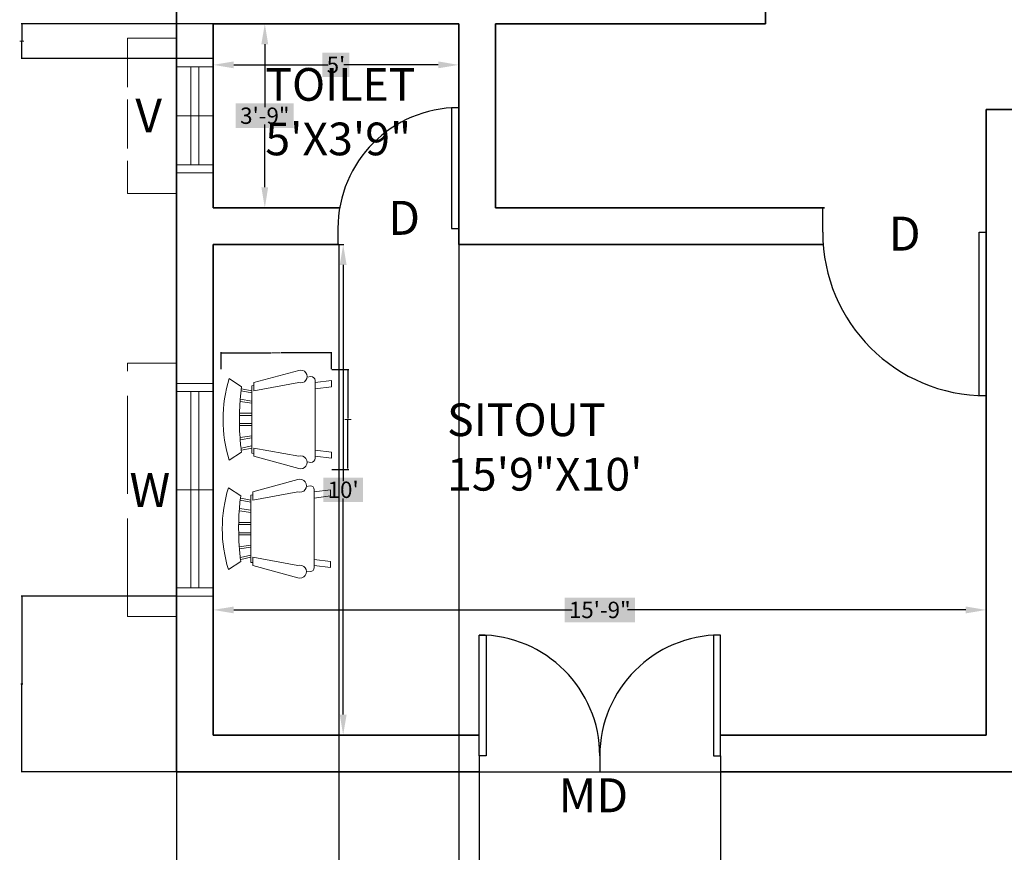
# Model space of a CAD drawing. Units: inches. Extents: x -128 to 854, y -395 to 398.
# Tile 22 of 61: x -88 to 152, y -109 to 95. Entities that reach past the tile are written whole.
import ezdxf

# ---------------------------------------------------------------- set-up
doc = ezdxf.new("R2010")
doc.units = ezdxf.units.IN
doc.header["$MEASUREMENT"] = 0
doc.linetypes.add('ACAD_ISO02W100', pattern=[15, 12, -3])
for name, color, linetype, lineweight in [('A-ANNO-DIMS', 2, 'Continuous', 18), ('A-ANNO-TEXT', 2, 'Continuous', 18), ('A-AREA-IDEN', 1, 'Continuous', 18), ('A-DOOR', 4, 'Continuous', 25), ('A-FURN', 8, 'Continuous', 18), ('A-GLAZ', 220, 'Continuous', 18), ('A-GLAZ-OVHD', 220, 'ACAD_ISO02W100', 13), ('A-WALL', 4, 'Continuous', 35)]:
    doc.layers.add(name, color=color, linetype=linetype, lineweight=lineweight)
doc.styles.get("Standard").update_dxf_attribs({"font": 'arial.ttf'})
doc.dimstyles.get("Standard").update_dxf_attribs({"dimtxt": 0.18, "dimasz": 0.18, "dimexe": 0.18, "dimexo": 0.0625, "dimgap": 0.09, "dimtad": 0, "dimtih": 1, "dimtoh": 1, "dimdec": 1, "dimzin": 0, "dimdsep": 46, "dimlunit": 4, "dimtxsty": 'Standard', "dimcen": 0.09, "dimclrd": 1, "dimclre": 2, "dimclrt": 6, "dimadec": 0, "dimazin": 0, "dimtfac": 1, "dimtdec": 1, "dimtofl": 0, "dimtmove": 0, "dimatfit": 3, "dimfxl": 1, "dimtfill": 2, "dimtfillclr": 3, "dimtolj": 1, "dimtzin": 0, "dimarcsym": 0})

# ---------------------------------------------------------------- blocks, each defined once
blk = doc.blocks.new('*U7')
for p, q in [((-750, 0), (-750, -100)), ((0, 0), (0, -100))]:
    blk.add_line(p, q)
blk.add_lwpolyline([(0, 0), (0, 750), (-43.75, 750), (-43.75, 0)], close=True)
blk.add_arc((0, 0), 750, 90, 180)
blk = doc.blocks.new('*U8')
for p, q in [((-40, 0), (-40, 6)), ((0, 0), (0, 6))]:
    blk.add_line(p, q)
blk.add_lwpolyline([(0, 0), (0, -40), (-1.75, -40), (-1.75, 0)], close=True)
blk.add_arc((0, 0), 40, 180, 270)
blk = doc.blocks.new('*U10')
for p, q in [((0, 0), (0, -100)), ((750, 0), (750, -100))]:
    blk.add_line(p, q)
blk.add_lwpolyline([(0, 0), (0, 750), (43.75, 750), (43.75, 0)], close=True)
blk.add_arc((0, 0), 750, 0, 90)
blk = doc.blocks.new('Chair - Rocking')
for p, q in [((-8, -4.5), (-10, -1.5)), ((8, -4.5), (10, -1.5)), ((-7.5, -4.5), (-7, -7)), ((-6.5, -7), (-7.02225, -4.43)), ((-4.5, -7), (-4.96674, -4.19951)), ((-4, -7), (-4.40532, -4.16272)), ((-1.5, -4.05012), (-1.5, -7)), ((-1, -7), (-1, -4.05012)), ((1, -7), (1, -4.04655)), ((1.5, -4.05012), (1.5, -7)), ((4, -7), (4.40187, -4.18694)), ((4.5, -7), (4.96761, -4.19437)), ((6.5, -7), (7, -4.4057)), ((7.5, -4.5), (7, -7)), ((-8.23428, -6.99939), (-8.3093, -7.47958)), ((-8.23041, -7), (8.23915, -7)), ((8.31071, -7.48854), (8.23449, -7.00073)), ((-9, -7.5), (-12, -18.49999)), ((-7, -7.5), (-9, -7.5)), ((-9, -18.49999), (-7, -7.5)), ((7, -7.5), (9, -7.5)), ((9, -18.49999), (7, -7.5)), ((9, -7.5), (12, -18.49999)), ((-10.36644, -20.64523), (-10.5, -21.49999)), ((10.5, -21.49999), (10.3575, -20.58798)), ((-9, -22.49999), (-9.5, -26.49999)), ((0, -22.49999), (-9.5, -22.49999)), ((-8, -26.49999), (-7.5, -22.49999)), ((0, -22.49999), (9.5, -22.49999)), ((8, -26.49999), (7.5, -22.49999)), ((9, -22.49999), (9.5, -26.49999)), ((-9.5, -26.49999), (-8, -26.49999)), ((9.5, -26.49999), (8, -26.49999))]:
    blk.add_line(p, q)
for centre, radius, start, end in [((0, -34.08333), 34.08333, 72.93847, 107.0615), ((0, -68.25004), 64.25, 93.92211, 97.15267), ((0, -68.25004), 64.25, 82.84733, 93.92211), ((-10.5, -18.99999), 1.58114, 161.5651, 18.43495), ((10.5, -18.99999), 1.58114, 161.5651, 18.43495), ((-9.5, -21.49999), 1, 180, 270), ((9.5, -21.49999), 1, 270, 0)]:
    blk.add_arc(centre, radius, start, end)
blk = doc.blocks.new('*D40')
at = {"layer": 'A-ANNO-DIMS', "color": 0, "lineweight": -2, "transparency": 16777216}
for p, q in [((-41.13, -80.2), (-41.13, -49.47)), ((-36.13, -49.65), (46.6, -49.65)), ((142.87, -49.65), (60.14, -49.65)), ((147.87, -80.2), (147.87, -49.47))]:
    blk.add_line(p, q, dxfattribs=at)
at = {"layer": 'A-ANNO-DIMS', "color": 0, "transparency": 16777216}
for points in [[(-36.13, -48.82), (-36.13, -50.49), (-41.13, -49.65)], [(142.87, -48.82), (142.87, -50.49), (147.87, -49.65)]]:
    blk.add_solid(points, dxfattribs=at)
at = {"layer": 'Defpoints', "color": 0, "transparency": 16777216}
for p in [(147.87, -49.65), (-41.13, -80.26), (147.87, -80.26)]:
    blk.add_point(p, dxfattribs=at)
at = {"layer": 'A-ANNO-DIMS', "color": 0, "transparency": 16777216, "insert": (53.37, -49.65), "char_height": 4, "attachment_point": 5, "bg_fill": 1, "box_fill_scale": 1.25, "bg_fill_color": 3, "bg_fill_transparency": 0}
blk.add_mtext('\\A1;15\'-9"', dxfattribs=at)
blk = doc.blocks.new('*D41')
at = {"layer": 'A-ANNO-DIMS', "color": 0, "lineweight": -2, "transparency": 16777216}
for p, q in [((-41.06, 39.74), (-9.19, 39.74)), ((-9.37, 34.74), (-9.37, -18.13)), ((-9.37, -75.26), (-9.37, -22.39)), ((-41.06, -80.26), (-9.19, -80.26))]:
    blk.add_line(p, q, dxfattribs=at)
at = {"layer": 'A-ANNO-DIMS', "color": 0, "transparency": 16777216}
for points in [[(-10.2, 34.74), (-8.53, 34.74), (-9.37, 39.74)], [(-10.2, -75.26), (-8.53, -75.26), (-9.37, -80.26)]]:
    blk.add_solid(points, dxfattribs=at)
at = {"layer": 'Defpoints', "color": 0, "transparency": 16777216}
for p in [(-41.13, 39.74), (-9.37, 39.74), (-41.13, -80.26)]:
    blk.add_point(p, dxfattribs=at)
at = {"layer": 'A-ANNO-DIMS', "color": 0, "transparency": 16777216, "insert": (-9.37, -20.26), "char_height": 4, "attachment_point": 5, "bg_fill": 1, "box_fill_scale": 1.25, "bg_fill_color": 3, "bg_fill_transparency": 0}
blk.add_mtext("\\A1;10'", dxfattribs=at)
blk = doc.blocks.new('*D44')
at = {"layer": 'A-ANNO-DIMS', "color": 0, "lineweight": -2, "transparency": 16777216}
for p, q in [((-41.06, 93.74), (-28.35, 93.74)), ((-28.53, 88.74), (-28.53, 73.37)), ((-28.53, 53.74), (-28.53, 69.11)), ((-41.06, 48.74), (-28.35, 48.74))]:
    blk.add_line(p, q, dxfattribs=at)
at = {"layer": 'A-ANNO-DIMS', "color": 0, "transparency": 16777216}
for points in [[(-29.37, 88.74), (-27.7, 88.74), (-28.53, 93.74)], [(-29.37, 53.74), (-27.7, 53.74), (-28.53, 48.74)]]:
    blk.add_solid(points, dxfattribs=at)
at = {"layer": 'Defpoints', "color": 0, "transparency": 16777216}
for p in [(-41.13, 93.74), (-28.53, 93.74), (-41.13, 48.74)]:
    blk.add_point(p, dxfattribs=at)
at = {"layer": 'A-ANNO-DIMS', "color": 0, "transparency": 16777216, "insert": (-28.53, 71.24), "char_height": 4, "attachment_point": 5, "bg_fill": 1, "box_fill_scale": 1.25, "bg_fill_color": 3, "bg_fill_transparency": 0}
blk.add_mtext('\\A1;3\'-9"', dxfattribs=at)
blk = doc.blocks.new('*D45')
at = {"layer": 'A-ANNO-DIMS', "color": 0, "lineweight": -2, "transparency": 16777216}
for p, q in [((-41.13, 93.68), (-41.13, 83.5)), ((18.87, 93.68), (18.87, 83.5)), ((-36.13, 83.68), (-13.06, 83.68)), ((13.87, 83.68), (-9.2, 83.68))]:
    blk.add_line(p, q, dxfattribs=at)
at = {"layer": 'A-ANNO-DIMS', "color": 0, "transparency": 16777216}
for points in [[(-36.13, 84.52), (-36.13, 82.85), (-41.13, 83.68)], [(13.87, 84.52), (13.87, 82.85), (18.87, 83.68)]]:
    blk.add_solid(points, dxfattribs=at)
at = {"layer": 'Defpoints', "color": 0, "transparency": 16777216}
for p in [(-41.13, 93.74), (18.87, 93.74), (18.87, 83.68)]:
    blk.add_point(p, dxfattribs=at)
at = {"layer": 'A-ANNO-DIMS', "color": 0, "transparency": 16777216, "insert": (-11.13, 83.68), "char_height": 4, "attachment_point": 5, "bg_fill": 1, "box_fill_scale": 1.25, "bg_fill_color": 3, "bg_fill_transparency": 0}
blk.add_mtext("\\A1;5'", dxfattribs=at)
blk = doc.blocks.new('WIN-48IN')
for p, q in [((9, 52), (0, 52)), ((9, 50), (0, 50)), ((3.5, 50), (3.5, 2)), ((5.5, 50), (5.5, 2)), ((9, 26), (0, 26)), ((9, 2), (0, 2)), ((9, 0), (0, 0))]:
    blk.add_line(p, q)
blk = doc.blocks.new('SHADE-48IN')
at = {"ltscale": 2}
for p, q in [((12, 62), (0, 62)), ((0, 0), (0, 62)), ((12, 57), (12, 62)), ((12, 5), (12, 0)), ((12, 0), (0, 0))]:
    blk.add_line(p, q, dxfattribs=at)
blk = doc.blocks.new('VENT-24IN')
for p, q in [((0, 0), (0, 9)), ((2, 0), (2, 9)), ((14, 0), (14, 9)), ((26, 0), (26, 9)), ((28, 0), (28, 9)), ((2, 5.5), (26, 5.5)), ((2, 3.5), (26, 3.5))]:
    blk.add_line(p, q)
blk = doc.blocks.new('SHADE-24IN')
for p, q in [((0, 0), (0, 12)), ((38, 12), (0, 12)), ((38, 0), (38, 12)), ((5, 0), (0, 0)), ((33, 0), (38, 0))]:
    blk.add_line(p, q)
blk = doc.blocks.new('*D83')
at = {"layer": 'A-ANNO-DIMS', "color": 2, "lineweight": -2, "transparency": 16777216}
for p, q in [((-39.24, 9.23), (-39.24, 13.4)), ((-12.24, 9.23), (-12.24, 13.4))]:
    blk.add_line(p, q, dxfattribs=at)
at = {"layer": 'A-ANNO-DIMS', "color": 1, "lineweight": -2, "transparency": 16777216}
for p, q in [((-39.06, 13.22), (-26.95, 13.22)), ((-12.42, 13.22), (-24.53, 13.22))]:
    blk.add_line(p, q, dxfattribs=at)
at = {"layer": 'A-ANNO-DIMS', "color": 1, "transparency": 16777216}
for points in [[(-39.06, 13.25), (-39.06, 13.19), (-39.24, 13.22)], [(-12.42, 13.25), (-12.42, 13.19), (-12.24, 13.22)]]:
    blk.add_solid(points, dxfattribs=at)
at = {"layer": 'Defpoints', "color": 0, "transparency": 16777216}
for p in [(-39.24, 13.22), (-39.24, 9.17), (-12.24, 9.17)]:
    blk.add_point(p, dxfattribs=at)
at = {"layer": 'A-ANNO-DIMS', "color": 6, "transparency": 16777216, "insert": (-25.74, 13.22), "char_height": 0.18, "attachment_point": 5, "bg_fill": 1, "box_fill_scale": 1.25, "bg_fill_color": 3, "bg_fill_transparency": 0}
blk.add_mtext('\\A1;ROCKER 2\'-3" TYP.', dxfattribs=at)
blk = doc.blocks.new('*D84')
at = {"layer": 'A-ANNO-DIMS', "color": 2, "lineweight": -2, "transparency": 16777216}
for p, q in [((-12.18, 9.17), (-8.01, 9.17)), ((-12.18, -15.26), (-8.01, -15.26))]:
    blk.add_line(p, q, dxfattribs=at)
at = {"layer": 'A-ANNO-DIMS', "color": 1, "lineweight": -2, "transparency": 16777216}
for p, q in [((-8.19, 8.99), (-8.19, -2.86)), ((-8.19, -15.08), (-8.19, -3.23))]:
    blk.add_line(p, q, dxfattribs=at)
at = {"layer": 'A-ANNO-DIMS', "color": 1, "transparency": 16777216}
for points in [[(-8.22, 8.99), (-8.16, 8.99), (-8.19, 9.17)], [(-8.22, -15.08), (-8.16, -15.08), (-8.19, -15.26)]]:
    blk.add_solid(points, dxfattribs=at)
at = {"layer": 'Defpoints', "color": 0, "transparency": 16777216}
for p in [(-12.24, 9.17), (-8.19, 9.17), (-12.24, -15.26)]:
    blk.add_point(p, dxfattribs=at)
at = {"layer": 'A-ANNO-DIMS', "color": 6, "transparency": 16777216, "insert": (-8.19, -3.05), "char_height": 0.18, "attachment_point": 5, "bg_fill": 1, "box_fill_scale": 1.25, "bg_fill_color": 3, "bg_fill_transparency": 0}
blk.add_mtext('\\A1;2\'-0 1/2" TYP.', dxfattribs=at)
blk = doc.blocks.new('*D99')
at = {"layer": 'A-ANNO-DIMS', "color": 2, "lineweight": -2, "transparency": 16777216}
for p, q in [((23.85, -89.32), (23.85, -127.24)), ((82.9, -89.32), (82.9, -127.24))]:
    blk.add_line(p, q, dxfattribs=at)
at = {"layer": 'A-ANNO-DIMS', "color": 1, "lineweight": -2, "transparency": 16777216}
for p, q in [((24.03, -127.06), (52.97, -127.06)), ((82.72, -127.06), (53.78, -127.06))]:
    blk.add_line(p, q, dxfattribs=at)
at = {"layer": 'A-ANNO-DIMS', "color": 1, "transparency": 16777216}
for points in [[(24.03, -127.03), (24.03, -127.09), (23.85, -127.06)], [(82.72, -127.03), (82.72, -127.09), (82.9, -127.06)]]:
    blk.add_solid(points, dxfattribs=at)
at = {"layer": 'Defpoints', "color": 0, "transparency": 16777216}
for p in [(23.85, -89.26), (82.9, -89.26), (82.9, -127.06)]:
    blk.add_point(p, dxfattribs=at)
at = {"layer": 'A-ANNO-DIMS', "color": 6, "transparency": 16777216, "insert": (53.37, -127.06), "char_height": 0.18, "attachment_point": 5, "bg_fill": 1, "box_fill_scale": 1.25, "bg_fill_color": 3, "bg_fill_transparency": 0}
blk.add_mtext('\\A1;4\'-11"', dxfattribs=at)
blk = doc.blocks.new('*D100')
at = {"layer": 'A-ANNO-DIMS', "color": 2, "lineweight": -2, "transparency": 16777216}
for p, q in [((-50.13, -89.32), (-50.13, -127.24)), ((23.85, -89.32), (23.85, -127.24))]:
    blk.add_line(p, q, dxfattribs=at)
at = {"layer": 'A-ANNO-DIMS', "color": 1, "lineweight": -2, "transparency": 16777216}
for p, q in [((-49.95, -127.06), (-13.47, -127.06)), ((23.67, -127.06), (-12.81, -127.06))]:
    blk.add_line(p, q, dxfattribs=at)
at = {"layer": 'A-ANNO-DIMS', "color": 1, "transparency": 16777216}
for points in [[(-49.95, -127.03), (-49.95, -127.09), (-50.13, -127.06)], [(23.67, -127.03), (23.67, -127.09), (23.85, -127.06)]]:
    blk.add_solid(points, dxfattribs=at)
at = {"layer": 'Defpoints', "color": 0, "transparency": 16777216}
for p in [(-50.13, -89.26), (23.85, -89.26), (23.85, -127.06)]:
    blk.add_point(p, dxfattribs=at)
at = {"layer": 'A-ANNO-DIMS', "color": 6, "transparency": 16777216, "insert": (-13.14, -127.06), "char_height": 0.18, "attachment_point": 5, "bg_fill": 1, "box_fill_scale": 1.25, "bg_fill_color": 3, "bg_fill_transparency": 0}
blk.add_mtext('\\A1;6\'-2"', dxfattribs=at)
blk = doc.blocks.new('*D102')
at = {"layer": 'A-ANNO-DIMS', "color": 2, "lineweight": -2, "transparency": 16777216}
for p, q in [((-10.39, 39.68), (-10.39, -127.24)), ((18.87, 39.68), (18.87, -127.24))]:
    blk.add_line(p, q, dxfattribs=at)
at = {"layer": 'A-ANNO-DIMS', "color": 1, "lineweight": -2, "transparency": 16777216}
for p, q in [((-10.21, -127.06), (3.7, -127.06)), ((18.69, -127.06), (4.78, -127.06))]:
    blk.add_line(p, q, dxfattribs=at)
at = {"layer": 'A-ANNO-DIMS', "color": 1, "transparency": 16777216}
for points in [[(-10.21, -127.03), (-10.21, -127.09), (-10.39, -127.06)], [(18.69, -127.03), (18.69, -127.09), (18.87, -127.06)]]:
    blk.add_solid(points, dxfattribs=at)
at = {"layer": 'Defpoints', "color": 0, "transparency": 16777216}
for p in [(-10.39, 39.74), (18.87, 39.74), (18.87, -127.06)]:
    blk.add_point(p, dxfattribs=at)
at = {"layer": 'A-ANNO-DIMS', "color": 6, "transparency": 16777216, "insert": (4.24, -127.06), "char_height": 0.18, "attachment_point": 5, "bg_fill": 1, "box_fill_scale": 1.25, "bg_fill_color": 3, "bg_fill_transparency": 0}
blk.add_mtext('\\A1;2\'-5 1/2"', dxfattribs=at)
blk = doc.blocks.new('*D109')
at = {"layer": 'A-ANNO-DIMS', "color": 2, "lineweight": -2, "transparency": 16777216}
for p, q in [((-41.19, 93.74), (-88.11, 93.74)), ((-41.19, 85.24), (-88.11, 85.24))]:
    blk.add_line(p, q, dxfattribs=at)
at = {"layer": 'A-ANNO-DIMS', "color": 1, "lineweight": -2, "transparency": 16777216}
for p, q in [((-87.93, 93.56), (-87.93, 89.67)), ((-87.93, 85.42), (-87.93, 89.31))]:
    blk.add_line(p, q, dxfattribs=at)
at = {"layer": 'A-ANNO-DIMS', "color": 1, "transparency": 16777216}
for points in [[(-87.96, 93.56), (-87.9, 93.56), (-87.93, 93.74)], [(-87.96, 85.42), (-87.9, 85.42), (-87.93, 85.24)]]:
    blk.add_solid(points, dxfattribs=at)
at = {"layer": 'Defpoints', "color": 0, "transparency": 16777216}
for p in [(-41.13, 93.74), (-87.93, 85.24), (-41.13, 85.24)]:
    blk.add_point(p, dxfattribs=at)
at = {"layer": 'A-ANNO-DIMS', "color": 6, "transparency": 16777216, "insert": (-87.93, 89.49), "char_height": 0.18, "attachment_point": 5, "bg_fill": 1, "box_fill_scale": 1.25, "bg_fill_color": 3, "bg_fill_transparency": 0}
blk.add_mtext('\\A1;0\'-8 1/2"', dxfattribs=at)
blk = doc.blocks.new('*D110')
at = {"layer": 'A-ANNO-DIMS', "color": 2, "lineweight": -2, "transparency": 16777216}
for p, q in [((-50.19, -46.26), (-88.11, -46.26)), ((-50.19, -89.26), (-88.11, -89.26))]:
    blk.add_line(p, q, dxfattribs=at)
at = {"layer": 'A-ANNO-DIMS', "color": 1, "lineweight": -2, "transparency": 16777216}
for p, q in [((-87.93, -46.44), (-87.93, -67.58)), ((-87.93, -89.08), (-87.93, -67.94))]:
    blk.add_line(p, q, dxfattribs=at)
at = {"layer": 'A-ANNO-DIMS', "color": 1, "transparency": 16777216}
for points in [[(-87.96, -46.44), (-87.9, -46.44), (-87.93, -46.26)], [(-87.96, -89.08), (-87.9, -89.08), (-87.93, -89.26)]]:
    blk.add_solid(points, dxfattribs=at)
at = {"layer": 'Defpoints', "color": 0, "transparency": 16777216}
for p in [(-87.93, -46.26), (-50.13, -46.26), (-50.13, -89.26)]:
    blk.add_point(p, dxfattribs=at)
at = {"layer": 'A-ANNO-DIMS', "color": 6, "transparency": 16777216, "insert": (-87.93, -67.76), "char_height": 0.18, "attachment_point": 5, "bg_fill": 1, "box_fill_scale": 1.25, "bg_fill_color": 3, "bg_fill_transparency": 0}
blk.add_mtext('\\A1;3\'-7"', dxfattribs=at)

msp = doc.modelspace()

# ---------------------------------------------------------------- linework, layer by layer
at = {"layer": 'A-DOOR'}
for p, q in [((53.37, -85.32), (53.37, -89.26)), ((23.85, -89.26), (82.9, -89.26))]:
    msp.add_line(p, q, dxfattribs=at)
at = {"layer": 'A-WALL'}
for p, q in [((-50.13, 156.74), (-50.13, 93.74)), ((93.87, 102.74), (93.87, 93.74)), ((-50.13, 93.74), (-50.13, 39.74)), ((-41.13, 93.74), (18.87, 93.74)), ((-41.13, 93.74), (-41.13, 48.74)), ((18.87, 39.74), (18.87, 93.74)), ((27.87, 48.74), (27.87, 93.74)), ((27.87, 93.74), (93.87, 93.74)), ((147.87, 72.74), (147.87, 48.74)), ((156.87, 72.74), (147.87, 72.74)), ((-41.13, 48.74), (-10.22, 48.74)), ((-10.22, 48.74), (-41.13, 48.74)), ((108.33, 48.74), (27.87, 48.74)), ((147.87, 48.69), (147.87, -80.26)), ((-50.13, 39.74), (-50.13, -89.26)), ((-41.13, 39.74), (-10.39, 39.74)), ((-41.13, 39.74), (-41.13, -80.26)), ((-10.39, 39.74), (-41.13, 39.74)), ((107.99, 39.74), (18.87, 39.74)), ((147.87, -80.26), (147.87, 39.74)), ((-41.13, -80.26), (23.85, -80.26)), ((82.9, -80.26), (147.87, -80.26)), ((-50.13, -89.26), (23.85, -89.26)), ((82.9, -89.26), (156.87, -89.26))]:
    msp.add_line(p, q, dxfattribs=at)

# ---------------------------------------------------------------- block references
at = {"layer": 'A-DOOR', "xscale": 0.0393700787401575, "yscale": 0.0393700787401575, "zscale": 0.0393700787401575}
for name, p in [('*U7', (18.87, 43.68)), ('*U10', (23.85, -85.32)), ('*U7', (82.9, -85.32))]:
    msp.add_blockref(name, p, dxfattribs=at)
at = {"layer": 'A-DOOR'}
msp.add_blockref('*U8', (147.87, 42.74), dxfattribs=at)
at = {"layer": 'A-FURN', "rotation": 90}
for p in [(-38.74, -3.05), (-38.93, -29.78)]:
    msp.add_blockref('Chair - Rocking', p, dxfattribs=at)
at = {"layer": 'A-GLAZ', "extrusion": (0, 0, -1), "zscale": -1}
for name, p, rotation in [('VENT-24IN', (50.13, 57.24), 89.99999999999953), ('WIN-48IN', (50.13, 5.74), 180)]:
    msp.add_blockref(name, p, dxfattribs=dict(at, rotation=rotation))
at = {"layer": 'A-GLAZ-OVHD', "rotation": 90.00000000000003}
msp.add_blockref('SHADE-24IN', (-50.13, 52.24), dxfattribs=at)
at = {"layer": 'A-GLAZ-OVHD'}
msp.add_blockref('SHADE-48IN', (-62.13, -51.26), dxfattribs=at)

# ---------------------------------------------------------------- texts
at = {"layer": 'A-ANNO-TEXT'}
for s, height, p in [('V', 8.31, (-60.19, 67.14)), ('D', 8.31, (1.63, 42.1)), ('D', 8.31, (124.02, 38.24)), ('W', 8.31, (-61.61, -24.49)), ('MD', 8.314, (43.29, -99.16))]:
    msp.add_text(s, height=height, dxfattribs=at).set_placement(p)
at = {"layer": 'A-AREA-IDEN', "char_height": 8, "attachment_point": 1}
for s, insert in [('TOILET\\P5\'X3\'9"', (-28.41, 82.9)), ('SITOUT\\P15\'9"X10\'', (16.04, 0.87))]:
    msp.add_mtext_dynamic_manual_height_columns(s, width=99.0352, gutter_width=1, heights=[0], dxfattribs=dict(at, insert=insert))

# ---------------------------------------------------------------- dimensions: what is measured, and where the dimension line sits
at = {"layer": 'A-ANNO-DIMS'}
for base, p1, p2, override, picture, middle in [((-87.93, 85.24), (-41.13, 93.74), (-41.13, 85.24), {"dimdec": 1, "dimlfac": 1, "dimrnd": 0, "dimzin": 1, "dimdsep": 46, "dimlunit": 4, "dimfrac": 2}, '*D109', (-87.93, 89.49)), ((-28.53, 93.74), (-41.13, 48.74), (-41.13, 93.74), {"dimtxt": 4, "dimasz": 5, "dimclrd": 0, "dimclre": 0, "dimclrt": 0}, '*D44', (-28.53, 71.24)), ((-9.37, 39.74), (-41.13, -80.26), (-41.13, 39.74), {"dimtxt": 4, "dimasz": 5, "dimclrd": 0, "dimclre": 0, "dimclrt": 0}, '*D41', (-9.37, -20.26)), ((-87.93, -46.26), (-50.13, -89.26), (-50.13, -46.26), {"dimdec": 1, "dimlfac": 1, "dimrnd": 0, "dimzin": 1, "dimdsep": 46, "dimlunit": 4, "dimfrac": 2}, '*D110', (-87.93, -67.76))]:
    dim = msp.add_linear_dim(base=base, p1=p1, p2=p2, angle=90, dimstyle='Standard', override=override, dxfattribs=at)
    dim.commit()
    dim.dimension.update_dxf_attribs({"geometry": picture, "text_midpoint": middle})
for base, p1, p2, override, picture, middle in [((18.87, 83.68), (-41.13, 93.74), (18.87, 93.74), {"dimtxt": 4, "dimasz": 5, "dimclrd": 0, "dimclre": 0, "dimclrt": 0}, '*D45', (-11.13, 83.68)), ((18.87, -127.06), (-10.39, 39.74), (18.87, 39.74), {"dimdec": 1, "dimlfac": 1, "dimrnd": 0, "dimzin": 1, "dimdsep": 46, "dimlunit": 4, "dimfrac": 2}, '*D102', (4.24, -127.06)), ((147.87, -49.65), (-41.13, -80.26), (147.87, -80.26), {"dimtxt": 4, "dimasz": 5, "dimclrd": 0, "dimclre": 0, "dimclrt": 0}, '*D40', (53.37, -49.65)), ((23.85, -127.06), (-50.13, -89.26), (23.85, -89.26), {"dimdec": 1, "dimlfac": 1, "dimrnd": 0, "dimzin": 1, "dimdsep": 46, "dimlunit": 4, "dimfrac": 2}, '*D100', (-13.14, -127.06)), ((82.9003, -127.0595), (23.8451, -89.2595), (82.9003, -89.2595), {"dimdec": 1, "dimlfac": 1, "dimrnd": 0, "dimzin": 1, "dimdsep": 46, "dimlunit": 4, "dimfrac": 2}, '*D99', (53.3727, -127.0595))]:
    dim = msp.add_linear_dim(base=base, p1=p1, p2=p2, dimstyle='Standard', override=override, dxfattribs=at)
    dim.commit()
    dim.dimension.update_dxf_attribs({"geometry": picture, "text_midpoint": middle})
for base, p1, p2, angle, text, picture, middle in [((-39.24, 13.22), (-12.24, 9.17), (-39.24, 9.17), 180, 'ROCKER <> TYP.', '*D83', (-25.74, 13.22)), ((-8.19, 9.17), (-12.24, -15.26), (-12.24, 9.17), 90, '<> TYP.', '*D84', (-8.19, -3.05))]:
    dim = msp.add_linear_dim(base=base, p1=p1, p2=p2, angle=angle, text=text, dimstyle='Standard', override={"dimdec": 1, "dimlfac": 1, "dimrnd": 0, "dimzin": 1, "dimdsep": 46, "dimlunit": 4, "dimfrac": 2}, dxfattribs=at)
    dim.commit()
    dim.dimension.update_dxf_attribs({"geometry": picture, "text_midpoint": middle})

doc.saveas('drawing.dxf')
